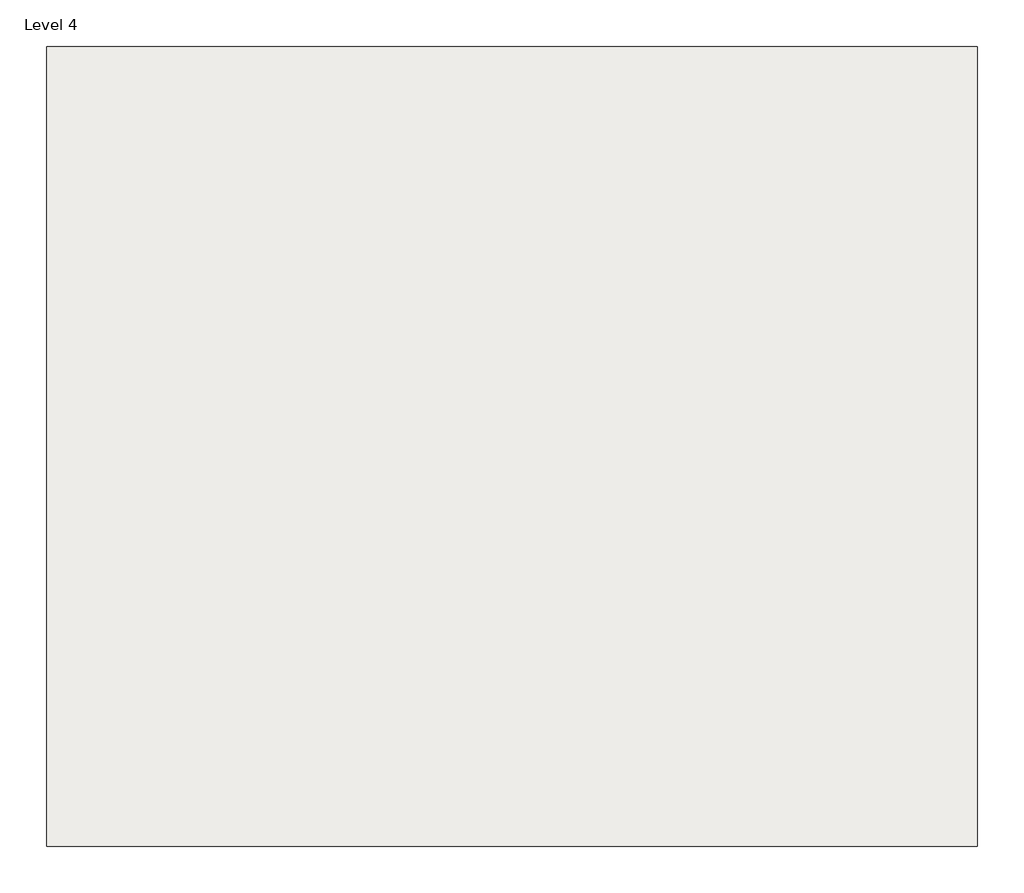
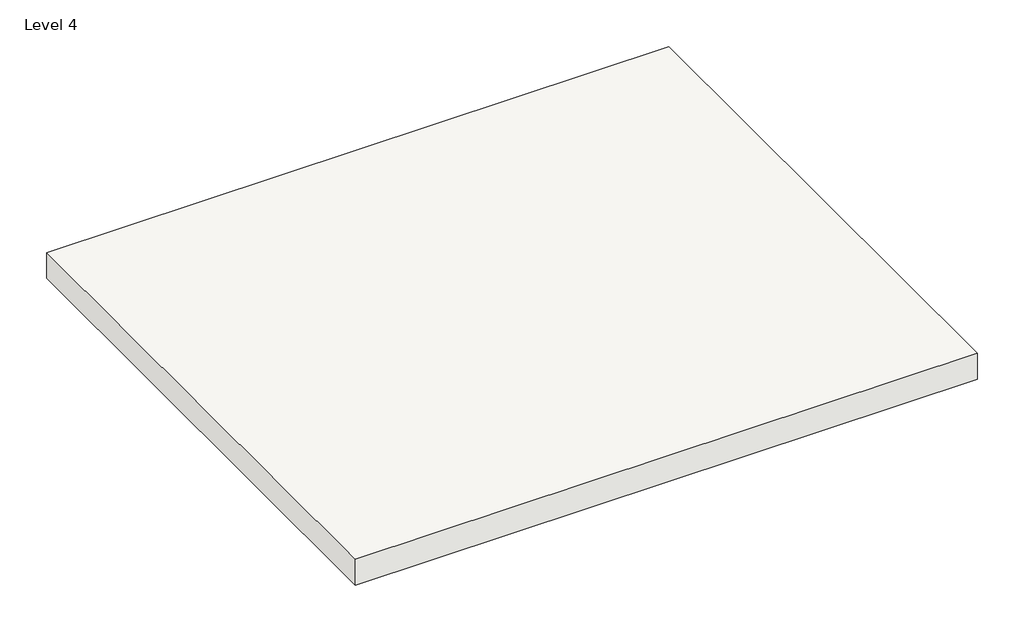
# One storey: 1 slab.
"""IFC4 building model written with IfcOpenShell, lengths in millimetres."""

from ifc_helpers import new_model, si_unit, frame, origin, place, context, project, spatial, polyline, outline, extrude, element, save

model = new_model("IFC4")

# Units and contexts
model_context = context("Model", 3, world=origin())
ifc_project = project(units=[si_unit("LENGTHUNIT", "METRE", prefix="MILLI")], contexts=[model_context])

# Site, building, storey
site = spatial("IfcSite", under=ifc_project)
building = spatial("IfcBuilding", under=site)
storey = spatial("IfcBuildingStorey", under=building, Name="Level 4", Elevation=9448.8)

# Slab
placement = place(None, origin())
element("IfcSlab", 1, ObjectType="6\"", at=placement, inside=storey, context=model_context, shape_type="SweptSolid", body=[
    extrude(outline(polyline([(-5735.8707895, 7858.9953048), (-5735.8707895, 4861.7953048), (-9222.6291271, 4861.7953048), (-9222.6291271, 7858.9953048), (-5735.8707895, 7858.9953048)])), frame((0.0, 0.0, 9448.8), z_axis=(0.0, 0.0, 1.0), x_axis=(1.0, 0.0, 0.0)), (0.0, 0.0, 1.0), 152.4),
])

save(model, "model.ifc")

# Revit data of these elements
# Type "6\""
#   Assembly Code = "B1010"
#   Function = 0
#   Layers, outside or top first: 0' - 6" "FLOOR" (function 1)
# Element 1 (IfcSlab, "6\"")
#   Height Offset From Level = 0' - 6"
#   Phase Created = New Construction
#   Materials on its faces: "FLOOR"
# Materials
#   "FLOOR": class "Generic", colour RGB 140 134 116, transparency 0, Cost = 0
